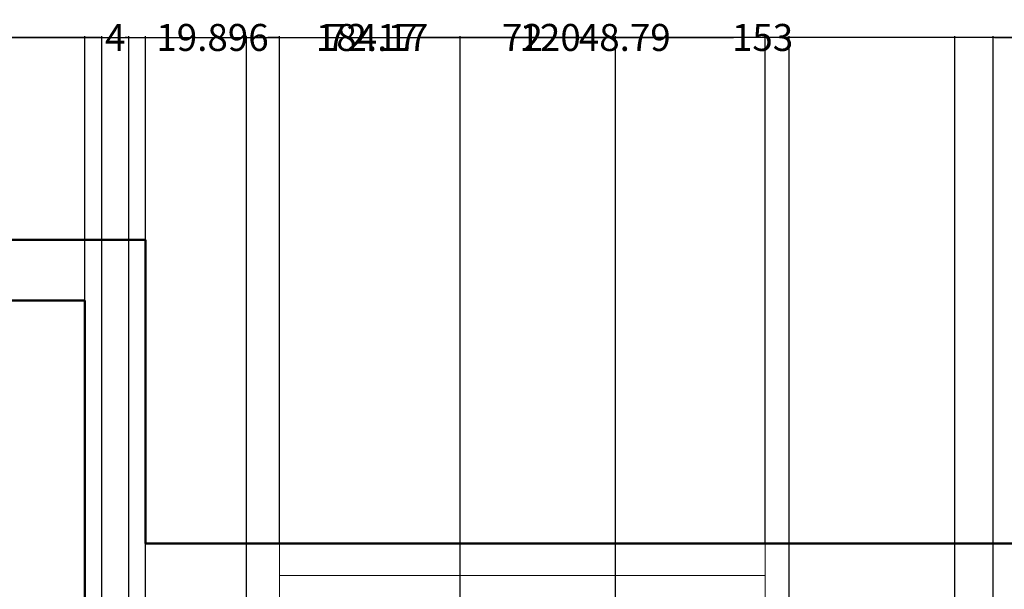
# Model space of a CAD drawing. Units: inches. Extents: x 1454 to 2136, y 626 to 1213.
# Tile 20 of 23: x 1741 to 1887, y 1128 to 1213. Entities that reach past the tile are written whole.
import ezdxf

# ---------------------------------------------------------------- set-up
doc = ezdxf.new("R2010")
doc.units = ezdxf.units.IN
doc.header["$MEASUREMENT"] = 0
for name, color, linetype, lineweight in [('A-ANNO-DIMS', 2, 'Continuous', 18), ('A-GLAZ', 4, 'Continuous', 18), ('A-WALL', 7, 'Continuous', 50)]:
    doc.layers.add(name, color=color, linetype=linetype, lineweight=lineweight)
doc.styles.get("Standard").update_dxf_attribs({"font": 'arial.ttf'})
doc.dimstyles.get("Standard").update_dxf_attribs({"dimtxt": 4, "dimasz": 0.18, "dimexe": 0.18, "dimexo": 0.0625, "dimgap": 0.09, "dimtad": 0, "dimtih": 1, "dimtoh": 1, "dimdec": 0, "dimrnd": 6, "dimzin": 0, "dimdsep": 46, "dimlunit": 3, "dimtxsty": 'Standard', "dimcen": 0.09, "dimadec": 0, "dimazin": 0, "dimtfac": 1, "dimtdec": 0, "dimtofl": 0, "dimtmove": 0, "dimatfit": 3, "dimfxl": 1, "dimtolj": 1, "dimtzin": 0, "dimarcsym": 0})

# ---------------------------------------------------------------- blocks, each defined once
blk = doc.blocks.new('*D29')
at = {"layer": 'A-ANNO-DIMS', "color": 0, "lineweight": -2, "transparency": 16777216}
for p, q in [((1546.56, 1171.34), (1546.56, 1210.46)), ((1546.74, 1210.28), (1644.02, 1210.28)), ((1750.38, 1210.28), (1653.09, 1210.28)), ((1750.56, 1171.34), (1750.56, 1210.46))]:
    blk.add_line(p, q, dxfattribs=at)
at = {"layer": 'A-ANNO-DIMS', "color": 0, "transparency": 16777216}
for points in [[(1546.74, 1210.31), (1546.74, 1210.25), (1546.56, 1210.28)], [(1750.38, 1210.31), (1750.38, 1210.25), (1750.56, 1210.28)]]:
    blk.add_solid(points, dxfattribs=at)
at = {"layer": 'Defpoints', "color": 0, "transparency": 16777216}
for p in [(1750.56, 1210.28), (1546.56, 1171.28), (1750.56, 1171.28)]:
    blk.add_point(p, dxfattribs=at)
at = {"layer": 'A-ANNO-DIMS', "color": 0, "transparency": 16777216, "insert": (1648.56, 1210.28), "char_height": 4, "attachment_point": 5}
blk.add_mtext('\\A1;204', dxfattribs=at)
blk = doc.blocks.new('*D31')
at = {"layer": 'A-ANNO-DIMS', "color": 0, "lineweight": -2, "transparency": 16777216}
for p, q in [((1759.56, 1126.34), (1759.56, 1210.46)), ((1759.74, 1210.28), (1815.24, 1210.28)), ((1879.38, 1210.28), (1823.87, 1210.28)), ((1879.56, 1126.34), (1879.56, 1210.46))]:
    blk.add_line(p, q, dxfattribs=at)
at = {"layer": 'A-ANNO-DIMS', "color": 0, "transparency": 16777216}
for points in [[(1759.74, 1210.31), (1759.74, 1210.25), (1759.56, 1210.28)], [(1879.38, 1210.31), (1879.38, 1210.25), (1879.56, 1210.28)]]:
    blk.add_solid(points, dxfattribs=at)
at = {"layer": 'Defpoints', "color": 0, "transparency": 16777216}
for p in [(1879.56, 1210.28), (1759.56, 1126.28), (1879.56, 1126.28)]:
    blk.add_point(p, dxfattribs=at)
at = {"layer": 'A-ANNO-DIMS', "color": 0, "transparency": 16777216, "insert": (1819.56, 1210.28), "char_height": 4, "attachment_point": 5}
blk.add_mtext('\\A1;120', dxfattribs=at)
blk = doc.blocks.new('*D37')
at = {"layer": 'A-ANNO-DIMS', "color": 0, "lineweight": -2, "transparency": 16777216}
for p, q in [((1774.56, 712.34), (1774.56, 1210.46)), ((1774.74, 1210.28), (1846.74, 1210.28)), ((1927.38, 1210.28), (1855.38, 1210.28)), ((1927.56, 712.34), (1927.56, 1210.46))]:
    blk.add_line(p, q, dxfattribs=at)
at = {"layer": 'A-ANNO-DIMS', "color": 0, "transparency": 16777216}
for points in [[(1774.74, 1210.31), (1774.74, 1210.25), (1774.56, 1210.28)], [(1927.38, 1210.31), (1927.38, 1210.25), (1927.56, 1210.28)]]:
    blk.add_solid(points, dxfattribs=at)
at = {"layer": 'Defpoints', "color": 0, "transparency": 16777216}
for p in [(1927.56, 1210.28), (1774.56, 712.28), (1927.56, 712.28)]:
    blk.add_point(p, dxfattribs=at)
at = {"layer": 'A-ANNO-DIMS', "color": 0, "transparency": 16777216, "insert": (1851.06, 1210.28), "char_height": 4, "attachment_point": 5}
blk.add_mtext('\\A1;153', dxfattribs=at)
blk = doc.blocks.new('*D44')
at = {"layer": 'A-ANNO-DIMS', "color": 0, "lineweight": -2, "transparency": 16777216}
for p, q in [((1701.08, 909.11), (1701.08, 1210.46)), ((1701.26, 1210.28), (1784.96, 1210.28)), ((1885.07, 1210.28), (1801.37, 1210.28)), ((1885.25, 909.11), (1885.25, 1210.46))]:
    blk.add_line(p, q, dxfattribs=at)
at = {"layer": 'A-ANNO-DIMS', "color": 0, "transparency": 16777216}
for points in [[(1701.26, 1210.31), (1701.26, 1210.25), (1701.08, 1210.28)], [(1885.07, 1210.31), (1885.07, 1210.25), (1885.25, 1210.28)]]:
    blk.add_solid(points, dxfattribs=at)
at = {"layer": 'Defpoints', "color": 0, "transparency": 16777216}
for p in [(1885.25, 1210.28), (1701.08, 909.05), (1885.25, 909.05)]:
    blk.add_point(p, dxfattribs=at)
at = {"layer": 'A-ANNO-DIMS', "color": 0, "transparency": 16777216, "insert": (1793.16, 1210.28), "char_height": 4, "attachment_point": 5}
blk.add_mtext('\\A1;184.17', dxfattribs=at)
blk = doc.blocks.new('*D47')
at = {"layer": 'A-ANNO-DIMS', "color": 0, "lineweight": -2, "transparency": 16777216}
for p, q in [((1885.25, 909.11), (1885.25, 1210.46)), ((1885.43, 1210.28), (1899.87, 1210.28)), ((1927.38, 1210.28), (1912.94, 1210.28)), ((1927.56, 910.34), (1927.56, 1210.46))]:
    blk.add_line(p, q, dxfattribs=at)
at = {"layer": 'A-ANNO-DIMS', "color": 0, "transparency": 16777216}
for points in [[(1885.43, 1210.31), (1885.43, 1210.25), (1885.25, 1210.28)], [(1927.38, 1210.31), (1927.38, 1210.25), (1927.56, 1210.28)]]:
    blk.add_solid(points, dxfattribs=at)
at = {"layer": 'Defpoints', "color": 0, "transparency": 16777216}
for p in [(1885.25, 1210.28), (1927.56, 910.28), (1885.25, 909.05)]:
    blk.add_point(p, dxfattribs=at)
at = {"layer": 'A-ANNO-DIMS', "color": 0, "transparency": 16777216, "insert": (1906.4, 1210.28), "char_height": 4, "attachment_point": 5}
blk.add_mtext('\\A1;42.31', dxfattribs=at)
blk = doc.blocks.new('*D59')
at = {"layer": 'A-ANNO-DIMS', "color": 0, "lineweight": -2, "transparency": 16777216}
for p, q in [((1779.45, 1135.31), (1779.45, 1210.46)), ((1779.63, 1210.28), (1812.53, 1210.28)), ((1851.27, 1210.28), (1818.37, 1210.28)), ((1851.45, 1135.31), (1851.45, 1210.46))]:
    blk.add_line(p, q, dxfattribs=at)
at = {"layer": 'A-ANNO-DIMS', "color": 0, "transparency": 16777216}
for points in [[(1779.63, 1210.31), (1779.63, 1210.25), (1779.45, 1210.28)], [(1851.27, 1210.31), (1851.27, 1210.25), (1851.45, 1210.28)]]:
    blk.add_solid(points, dxfattribs=at)
at = {"layer": 'Defpoints', "color": 0, "transparency": 16777216}
for p in [(1851.45, 1210.28), (1779.45, 1135.25), (1851.45, 1135.25)]:
    blk.add_point(p, dxfattribs=at)
at = {"layer": 'A-ANNO-DIMS', "color": 0, "transparency": 16777216, "insert": (1815.45, 1210.28), "char_height": 4, "attachment_point": 5}
blk.add_mtext('\\A1;72', dxfattribs=at)
blk = doc.blocks.new('*D60')
at = {"layer": 'A-ANNO-DIMS', "color": 0, "lineweight": -2, "transparency": 16777216}
for p, q in [((1759.56, 1135.34), (1759.56, 1210.46)), ((1759.74, 1210.28), (1761.3, 1210.28)), ((1779.27, 1210.28), (1777.71, 1210.28)), ((1779.45, 1135.31), (1779.45, 1210.46))]:
    blk.add_line(p, q, dxfattribs=at)
at = {"layer": 'A-ANNO-DIMS', "color": 0, "transparency": 16777216}
for points in [[(1759.74, 1210.31), (1759.74, 1210.25), (1759.56, 1210.28)], [(1779.27, 1210.31), (1779.27, 1210.25), (1779.45, 1210.28)]]:
    blk.add_solid(points, dxfattribs=at)
at = {"layer": 'Defpoints', "color": 0, "transparency": 16777216}
for p in [(1779.45, 1210.28), (1759.56, 1135.28), (1779.45, 1135.25)]:
    blk.add_point(p, dxfattribs=at)
at = {"layer": 'A-ANNO-DIMS', "color": 0, "transparency": 16777216, "insert": (1769.5, 1210.28), "char_height": 4, "attachment_point": 5}
blk.add_mtext('\\A1;19.896', dxfattribs=at)
blk = doc.blocks.new('*D66')
at = {"layer": 'A-ANNO-DIMS', "color": 0, "lineweight": -2, "transparency": 16777216}
for p, q in [((1757.08, 771.01), (1757.08, 1210.46)), ((1757.26, 1210.28), (1786.34, 1210.28)), ((1829.07, 1210.28), (1799.99, 1210.28)), ((1829.25, 771.01), (1829.25, 1210.46))]:
    blk.add_line(p, q, dxfattribs=at)
at = {"layer": 'A-ANNO-DIMS', "color": 0, "transparency": 16777216}
for points in [[(1757.26, 1210.31), (1757.26, 1210.25), (1757.08, 1210.28)], [(1829.07, 1210.31), (1829.07, 1210.25), (1829.25, 1210.28)]]:
    blk.add_solid(points, dxfattribs=at)
at = {"layer": 'Defpoints', "color": 0, "transparency": 16777216}
for p in [(1829.25, 1210.28), (1757.08, 770.95), (1829.25, 770.95)]:
    blk.add_point(p, dxfattribs=at)
at = {"layer": 'A-ANNO-DIMS', "color": 0, "transparency": 16777216, "insert": (1793.16, 1210.28), "char_height": 4, "attachment_point": 5}
blk.add_mtext('\\A1;72.17', dxfattribs=at)
blk = doc.blocks.new('*D69')
at = {"layer": 'A-ANNO-DIMS', "color": 0, "lineweight": -2, "transparency": 16777216}
for p, q in [((1806.23, 1089.59), (1806.23, 1210.46)), ((1806.41, 1210.28), (1823.7, 1210.28)), ((1854.84, 1210.28), (1837.55, 1210.28)), ((1855.02, 1089.59), (1855.02, 1210.46))]:
    blk.add_line(p, q, dxfattribs=at)
at = {"layer": 'A-ANNO-DIMS', "color": 0, "transparency": 16777216}
for points in [[(1806.41, 1210.31), (1806.41, 1210.25), (1806.23, 1210.28)], [(1854.84, 1210.31), (1854.84, 1210.25), (1855.02, 1210.28)]]:
    blk.add_solid(points, dxfattribs=at)
at = {"layer": 'Defpoints', "color": 0, "transparency": 16777216}
for p in [(1855.02, 1210.28), (1806.23, 1089.52), (1855.02, 1089.52)]:
    blk.add_point(p, dxfattribs=at)
at = {"layer": 'A-ANNO-DIMS', "color": 0, "transparency": 16777216, "insert": (1830.63, 1210.28), "char_height": 4, "attachment_point": 5}
blk.add_mtext('\\A1;48.79', dxfattribs=at)
blk = doc.blocks.new('*D77')
at = {"layer": 'A-ANNO-DIMS', "color": 0, "lineweight": -2, "transparency": 16777216}
for p, q in [((1753.08, 771.01), (1753.08, 1210.46)), ((1753.26, 1210.28), (1753.6, 1210.28)), ((1756.9, 1210.28), (1756.55, 1210.28)), ((1757.08, 771.01), (1757.08, 1210.46))]:
    blk.add_line(p, q, dxfattribs=at)
at = {"layer": 'A-ANNO-DIMS', "color": 0, "transparency": 16777216}
for points in [[(1753.26, 1210.31), (1753.26, 1210.25), (1753.08, 1210.28)], [(1756.9, 1210.31), (1756.9, 1210.25), (1757.08, 1210.28)]]:
    blk.add_solid(points, dxfattribs=at)
at = {"layer": 'Defpoints', "color": 0, "transparency": 16777216}
for p in [(1757.08, 1210.28), (1753.08, 770.95), (1757.08, 770.95)]:
    blk.add_point(p, dxfattribs=at)
at = {"layer": 'A-ANNO-DIMS', "color": 0, "transparency": 16777216, "insert": (1755.08, 1210.28), "char_height": 4, "attachment_point": 5}
blk.add_mtext('\\A1;4', dxfattribs=at)
blk = doc.blocks.new('*D78')
at = {"layer": 'A-ANNO-DIMS', "color": 0, "lineweight": -2, "transparency": 16777216}
for p, q in [((1705.08, 833.11), (1705.08, 1210.46)), ((1705.26, 1210.28), (1726.04, 1210.28)), ((1752.9, 1210.28), (1732.12, 1210.28)), ((1753.08, 833.11), (1753.08, 1210.46))]:
    blk.add_line(p, q, dxfattribs=at)
at = {"layer": 'A-ANNO-DIMS', "color": 0, "transparency": 16777216}
for points in [[(1705.26, 1210.31), (1705.26, 1210.25), (1705.08, 1210.28)], [(1752.9, 1210.31), (1752.9, 1210.25), (1753.08, 1210.28)]]:
    blk.add_solid(points, dxfattribs=at)
at = {"layer": 'Defpoints', "color": 0, "transparency": 16777216}
for p in [(1753.08, 1210.28), (1705.08, 833.05), (1753.08, 833.05)]:
    blk.add_point(p, dxfattribs=at)
at = {"layer": 'A-ANNO-DIMS', "color": 0, "transparency": 16777216, "insert": (1729.08, 1210.28), "char_height": 4, "attachment_point": 5}
blk.add_mtext('\\A1;48', dxfattribs=at)
blk = doc.blocks.new('*D81')
at = {"layer": 'A-ANNO-DIMS', "color": 0, "lineweight": -2, "transparency": 16777216}
for p, q in [((1701.82, 1088.13), (1701.82, 1210.46)), ((1702, 1210.28), (1719.28, 1210.28)), ((1750.38, 1210.28), (1733.1, 1210.28)), ((1750.56, 1027.34), (1750.56, 1210.46))]:
    blk.add_line(p, q, dxfattribs=at)
at = {"layer": 'A-ANNO-DIMS', "color": 0, "transparency": 16777216}
for points in [[(1702, 1210.31), (1702, 1210.25), (1701.82, 1210.28)], [(1750.38, 1210.31), (1750.38, 1210.25), (1750.56, 1210.28)]]:
    blk.add_solid(points, dxfattribs=at)
at = {"layer": 'Defpoints', "color": 0, "transparency": 16777216}
for p in [(1701.82, 1210.28), (1701.82, 1088.07), (1750.56, 1027.28)]:
    blk.add_point(p, dxfattribs=at)
at = {"layer": 'A-ANNO-DIMS', "color": 0, "transparency": 16777216, "insert": (1726.19, 1210.28), "char_height": 4, "attachment_point": 5}
blk.add_mtext('\\A1;48.74', dxfattribs=at)

msp = doc.modelspace()

# ---------------------------------------------------------------- linework, layer by layer
at = {"layer": 'A-GLAZ'}
msp.add_line((1851.4527, 1130.5527), (1779.4527, 1130.5527), dxfattribs=at)
msp.add_lwpolyline([(1779.4527, 1135.2472), (1851.4527, 1135.2472), (1851.4527, 1126.2472), (1779.4527, 1126.2472)], close=True, dxfattribs=at)
at = {"layer": 'A-WALL'}
for p, q in [((1759.5563, 1180.2825), (1537.5563, 1180.2825)), ((1759.5563, 1180.2825), (1759.5563, 1135.2825)), ((1750.5563, 1171.2825), (1546.5563, 1171.2825)), ((1750.5563, 1171.2825), (1750.5563, 1027.2825)), ((2041.5563, 1135.2825), (1759.5563, 1135.2825))]:
    msp.add_line(p, q, dxfattribs=at)

# ---------------------------------------------------------------- dimensions: what is measured, and where the dimension line sits
at = {"layer": 'A-ANNO-DIMS'}
for base, p1, p2, override, picture, middle in [((1750.5563, 1210.2845), (1546.5563, 1171.2825), (1750.5563, 1171.2825), {"dimdec": 0, "dimlfac": 1, "dimrnd": 0, "dimzin": 0, "dimdsep": 46, "dimlunit": 2}, '*D29', (1648.5563, 1210.2845)), ((1885.2497, 1210.2845), (1701.0763, 909.0476), (1885.2497, 909.0476), {"dimdec": 2, "dimlfac": 1, "dimrnd": 0, "dimzin": 0, "dimdsep": 46, "dimlunit": 2}, '*D44', (1793.163, 1210.2845)), ((1701.8177, 1210.2845), (1750.5563, 1027.2825), (1701.8177, 1088.0655), {"dimdec": 2, "dimlfac": 1, "dimrnd": 0, "dimzin": 0, "dimdsep": 46, "dimlunit": 2}, '*D81', (1726.187, 1210.2845)), ((1753.0763, 1210.2845), (1705.0763, 833.0476), (1753.0763, 833.0476), {"dimdec": 0, "dimlfac": 1, "dimrnd": 0, "dimzin": 0, "dimdsep": 46, "dimlunit": 2}, '*D78', (1729.0763, 1210.2845)), ((1757.0763, 1210.2845), (1753.0763, 770.9473), (1757.0763, 770.9473), {"dimdec": 0, "dimlfac": 1, "dimrnd": 0, "dimzin": 0, "dimdsep": 46, "dimlunit": 2}, '*D77', (1755.0763, 1210.2845)), ((1829.2497, 1210.2845), (1757.0763, 770.9473), (1829.2497, 770.9473), {"dimdec": 2, "dimlfac": 1, "dimrnd": 0, "dimzin": 0, "dimdsep": 46, "dimlunit": 2}, '*D66', (1793.163, 1210.2845)), ((1879.5563, 1210.2845), (1759.5563, 1126.2825), (1879.5563, 1126.2825), {"dimdec": 0, "dimlfac": 1, "dimrnd": 0, "dimzin": 0, "dimdsep": 46, "dimlunit": 2}, '*D31', (1819.5563, 1210.2845)), ((1779.4527, 1210.2845), (1759.5563, 1135.2825), (1779.4527, 1135.2472), {"dimdec": 3, "dimlfac": 1, "dimrnd": 0, "dimzin": 0, "dimdsep": 46, "dimlunit": 2}, '*D60', (1769.5045, 1210.2845)), ((1927.5563, 1210.2845), (1774.5563, 712.2825), (1927.5563, 712.2825), {"dimdec": 0, "dimlfac": 1, "dimrnd": 0, "dimzin": 0, "dimdsep": 46, "dimlunit": 2}, '*D37', (1851.0563, 1210.2845)), ((1851.4527, 1210.2845), (1779.4527, 1135.2472), (1851.4527, 1135.2472), {"dimdec": 0, "dimlfac": 1, "dimrnd": 0, "dimzin": 0, "dimdsep": 46, "dimlunit": 2}, '*D59', (1815.4527, 1210.2845)), ((1855.0231, 1210.2845), (1806.2288, 1089.5248), (1855.0231, 1089.5248), {"dimdec": 2, "dimlfac": 1, "dimrnd": 0, "dimzin": 0, "dimdsep": 46, "dimlunit": 2}, '*D69', (1830.626, 1210.2845)), ((1885.2497, 1210.2845), (1927.5563, 910.2825), (1885.2497, 909.0476), {"dimdec": 2, "dimlfac": 1, "dimrnd": 0, "dimzin": 0, "dimdsep": 46, "dimlunit": 2}, '*D47', (1906.403, 1210.2845))]:
    dim = msp.add_linear_dim(base=base, p1=p1, p2=p2, dimstyle='Standard', override=override, dxfattribs=at)
    dim.commit()
    dim.dimension.update_dxf_attribs({"geometry": picture, "text_midpoint": middle})

doc.saveas('drawing.dxf')
